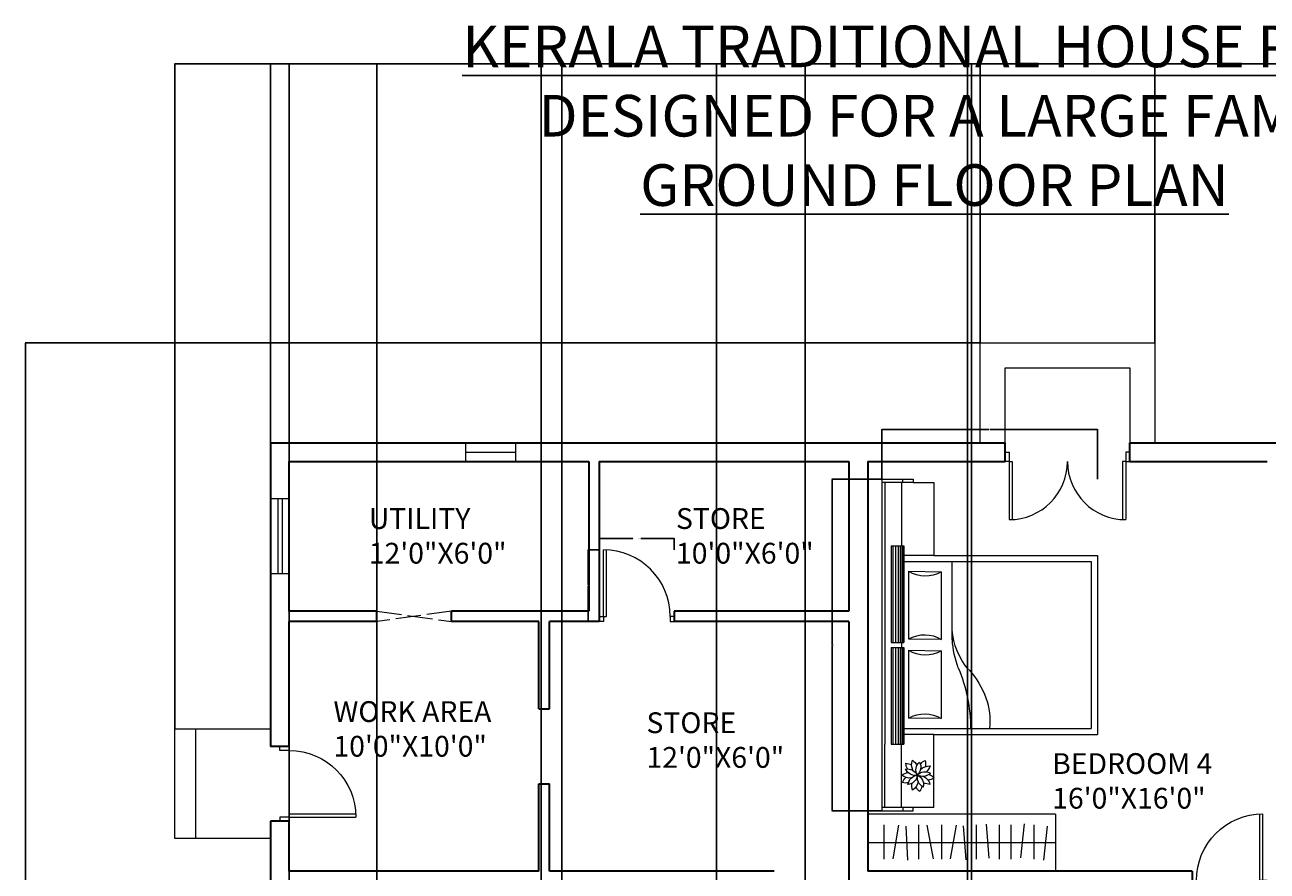
# Model space of a CAD drawing. Units: inches. Extents: x 4602 to 5612, y 5125 to 6591.
# Tile 5 of 6: x 4602 to 5199, y 6185 to 6591. Entities that reach past the tile are written whole.
import ezdxf

# ---------------------------------------------------------------- set-up
doc = ezdxf.new("R2010")
doc.units = ezdxf.units.IN
doc.linetypes.add('ACAD_ISO02W100', pattern=[15, 12, -3])
for name, color, linetype, lineweight in [('A-ANNO-DIMS', 2, 'Continuous', 18), ('A-ANNO-TEXT', 7, 'Continuous', 25), ('A-AREA-IDEN', 7, 'Continuous', 18), ('A-DOOR', 4, 'Continuous', 18), ('A-FLOR-CASE', 9, 'Continuous', 18), ('A-FLOR-STRS', 7, 'Continuous', 18), ('A-FURN', 8, 'Continuous', 13), ('A-GLAZ', 4, 'Continuous', 18), ('A-WALL', 7, 'Continuous', 35), ('A-WALL-OVHD', 8, 'ACAD_ISO02W100', 13)]:
    doc.layers.add(name, color=color, linetype=linetype, lineweight=lineweight)
doc.styles.get("Standard").update_dxf_attribs({"font": 'arial.ttf'})
doc.dimstyles.get("Standard").update_dxf_attribs({"dimtxt": 0.18, "dimasz": 0.18, "dimexe": 0.18, "dimexo": 0.0625, "dimgap": 0.09, "dimtad": 0, "dimtih": 1, "dimtoh": 1, "dimdec": 4, "dimzin": 0, "dimdsep": 46, "dimtxsty": 'Standard', "dimcen": 0.09, "dimadec": 0, "dimazin": 0, "dimtfac": 1, "dimtdec": 4, "dimtofl": 0, "dimtmove": 0, "dimatfit": 3, "dimfxl": 1, "dimtolj": 1, "dimtzin": 0, "dimarcsym": 0})

# ---------------------------------------------------------------- blocks, each defined once
blk = doc.blocks.new('A$C7BDD1693')
for p, q in [((0, 2.068), (0, 1.768)), ((0, 2.068), (1.615, 2.068)), ((0.03, 1.768), (0.03, 2.068)), ((0.03, 2.038), (0.64, 2.038)), ((0.64, 2.038), (1.565, 2.038)), ((1.565, 2.038), (1.615, 2.038)), ((1.615, 2.068), (2.54, 2.068)), ((1.615, 2.038), (2.54, 2.038)), ((2.54, 2.068), (3.18, 2.068)), ((3.15, 2.038), (2.54, 2.038)), ((3.15, 1.768), (3.15, 2.068)), ((3.18, 2.068), (3.18, 1.768)), ((0.64, 1.978), (1.565, 1.978)), ((0.64, 1.978), (0.64, 1.858)), ((0.64, 1.963), (1.565, 1.963)), ((0.64, 1.937), (1.565, 1.937)), ((0.64, 1.912), (1.565, 1.912)), ((1.565, 1.978), (1.565, 1.858)), ((1.615, 1.978), (1.615, 1.858)), ((1.615, 1.978), (2.54, 1.978)), ((1.615, 1.963), (2.54, 1.963)), ((1.615, 1.937), (2.54, 1.937)), ((1.615, 1.912), (2.54, 1.912)), ((2.54, 1.978), (2.54, 1.858)), ((0.03, 1.868), (0, 1.868)), ((0.03, 1.88), (0.64, 1.88)), ((0.64, 1.893), (1.565, 1.893)), ((0.64, 1.877), (1.565, 1.877)), ((0.64, 1.866), (1.565, 1.866)), ((0.64, 1.858), (1.565, 1.858)), ((0.73, 1.568), (0.73, 1.858)), ((0.79, 1.858), (0.79, 0.06)), ((1.533, 1.81), (0.883, 1.81)), ((0.883, 1.81), (0.887, 1.498)), ((1.537, 1.498), (1.533, 1.81)), ((1.565, 1.88), (1.615, 1.88)), ((1.615, 1.893), (2.54, 1.893)), ((1.615, 1.877), (2.54, 1.877)), ((1.615, 1.866), (2.54, 1.866)), ((1.615, 1.858), (2.54, 1.858)), ((2.291, 1.81), (1.641, 1.81)), ((1.641, 1.81), (1.646, 1.498)), ((2.296, 1.498), (2.291, 1.81)), ((2.39, 1.858), (2.39, 0.06)), ((2.45, 1.568), (2.45, 1.858)), ((3.15, 1.88), (2.54, 1.88)), ((3.15, 1.868), (3.18, 1.868)), ((0, 1.768), (0.03, 1.768)), ((0.03, 1.768), (0.03, 1.568)), ((0.03, 1.768), (0.03, 1.568)), ((3.15, 1.568), (3.15, 1.768)), ((3.18, 1.768), (3.15, 1.768)), ((0.03, 1.568), (0.73, 1.568)), ((0.73, 1.568), (0.73, 0)), ((3.15, 1.568), (2.45, 1.568)), ((2.45, 1.568), (2.45, 0)), ((0.887, 1.498), (1.537, 1.498)), ((1.646, 1.498), (2.296, 1.498)), ((1.54, 1.392), (0.79, 1.392)), ((1.848, 1.209), (0.79, 1.209)), ((0.73, 0), (2.45, 0)), ((0.79, 0.06), (2.39, 0.06))]:
    blk.add_line(p, q)
for centre, radius, start, end in [((0.626, 1.65), 0.303, 329.8722, 31.8713), ((1.794, 1.658), 0.303, 149.8722, 211.8713), ((1.384, 1.65), 0.303, 329.8722, 31.8713), ((2.553, 1.658), 0.303, 149.8722, 211.8713), ((2.879, 1.849), 0.155, 184.2105, 205.3514), ((2.726, 1.74), 0.0968, 57.5086, 91.2476), ((2.884, 1.823), 0.106, 170.7761, 244.5159), ((2.743, 1.749), 0.098, 347.0447, 68.2473), ((2.938, 1.802), 0.125, 143.1301, 173.4932), ((2.751, 1.802), 0.115, 351.1324, 40.6013), ((2.944, 1.713), 0.106, 98.7761, 172.5159), ((2.83, 1.825), 0.098, 275.0447, 356.2473), ((2.967, 1.726), 0.155, 112.2105, 133.3514), ((2.817, 1.838), 0.0968, 345.5086, 19.2476), ((2.74, 1.667), 0.115, 63.1324, 112.6013), ((2.798, 1.845), 0.125, 215.1301, 245.4931), ((2.791, 1.624), 0.0968, 129.5086, 163.2476), ((2.788, 1.643), 0.098, 59.0447, 140.2473), ((2.761, 1.8), 0.106, 242.7761, 316.5159), ((2.865, 1.615), 0.115, 135.1324, 184.6013), ((2.903, 1.653), 0.098, 131.0447, 212.2473), ((2.745, 1.676), 0.106, 314.7761, 28.5159), ((2.858, 1.622), 0.106, 26.7761, 100.5159), ((2.929, 1.765), 0.098, 203.0447, 284.2473), ((2.883, 1.833), 0.115, 279.1324, 328.6013), ((2.802, 1.607), 0.125, 359.1301, 29.4932), ((2.941, 1.655), 0.125, 71.1301, 101.4931), ((2.937, 1.782), 0.0968, 273.5086, 307.2476), ((2.877, 1.605), 0.155, 40.2105, 61.3514), ((2.735, 1.803), 0.155, 256.2105, 277.3514), ((2.713, 1.725), 0.125, 287.1301, 317.4932), ((2.921, 1.65), 0.0968, 201.5086, 235.2476), ((2.953, 1.718), 0.115, 207.1324, 256.6013), ((2.734, 1.652), 0.155, 328.2105, 349.3514)]:
    blk.add_arc(centre, radius, start, end)
for centre, major_axis, ratio, start_param, end_param in [((1.413, 0.552), (0, -0.842), 0.84, 2.512571, 3.097265), ((1.474, 0.023), (0, -1.371), 0.84, 2.845884, 3.083884), ((2.394, 3.329), (0, -2.112), 0.84, -0.336035, -0.002349), ((2.261, 1.856), (0.259, -0.793), 0.868451, -0.988378, -0.183496)]:
    blk.add_ellipse(centre, major_axis=major_axis, ratio=ratio, start_param=start_param, end_param=end_param)
blk = doc.blocks.new('DOOR-PAIR-60IN')
for p, q in [((2, 4.5), (2, 32.5)), ((3.5, 4.5), (3.5, 32.46)), ((56.5, 4.5), (56.5, 32.46)), ((58, 4.5), (58, 32.5)), ((2, 4.5), (0, 4.5)), ((2, 0), (2, 4.5)), ((2, 4.5), (3.5, 4.5)), ((58, 4.5), (56.5, 4.5)), ((58, 0), (58, 4.5)), ((58, 4.5), (60, 4.5)), ((0, 0), (2, 0)), ((60, 0), (58, 0))]:
    blk.add_line(p, q)
for centre, start, end in [((2, 4.5), 0, 90), ((58, 4.5), 90, 180)]:
    blk.add_arc(centre, 28, start, end)
blk = doc.blocks.new('DOOR-36IN-DEEP-JAMB')
for p, q in [((2, 4.5), (2, 36.5)), ((3.5, 4.5), (3.5, 36.46)), ((0, 4.5), (2, 4.5)), ((2, 4.5), (2, 0)), ((2, 4.5), (3.5, 4.5)), ((36, 4.5), (34, 4.5)), ((34, 4.5), (34, 0)), ((2, 0), (0, 0)), ((34, 0), (36, 0))]:
    blk.add_line(p, q)
blk.add_arc((2, 4.5), 32, 0, 90)
blk = doc.blocks.new('DOOR-36IN-SHALLOW-JAMB')
for p, q in [((2, 2.5), (2, 34.5)), ((3.5, 2.5), (3.5, 34.46)), ((0, 2.5), (2, 2.5)), ((2, 2.5), (2, 0)), ((2, 2.5), (3.5, 2.5)), ((36, 2.5), (34, 2.5)), ((34, 2.5), (34, 0)), ((2, 0), (0, 0)), ((34, 0), (36, 0))]:
    blk.add_line(p, q)
blk.add_arc((2, 2.5), 32, 0, 90)
blk = doc.blocks.new('WARDROBE-RAIL')
for p, q in [((90.22, 0), (90.22, 27.46)), ((3.99, 5.88), (5.71, 22.16)), ((10.39, 5.25), (10.39, 21.62)), ((15.01, 4.71), (16.73, 21)), ((21.48, 5.25), (21.48, 21.62)), ((27.02, 5.25), (27.02, 21.62)), ((33.26, 4.83), (31.94, 21.15)), ((38.1, 5.25), (38.1, 21.62)), ((44.31, 5.72), (42.98, 22.05)), ((47.72, 5.36), (50.53, 21.49)), ((54.72, 5.25), (54.72, 21.62)), ((61.87, 5.4), (58.77, 21.48)), ((65.8, 5.25), (65.8, 21.62)), ((70.89, 22.2), (71.76, 5.85)), ((75.49, 5.36), (78.19, 21.52)), ((82.43, 5.25), (82.43, 21.62)), ((90.22, 13.73), (0, 13.73)), ((0, 0), (90.22, 0))]:
    blk.add_line(p, q)
blk = doc.blocks.new('*D25')
at = {"layer": 'A-ANNO-DIMS', "color": 0, "lineweight": -2, "transparency": 16777216}
for p, q in [((4878.24, 6339.11), (4878.24, 6344.63)), ((4878.42, 6344.45), (4894.27, 6344.45)), ((4914.06, 6344.45), (4898.21, 6344.45)), ((4914.24, 6339.11), (4914.24, 6344.63))]:
    blk.add_line(p, q, dxfattribs=at)
at = {"layer": 'A-ANNO-DIMS', "color": 0, "transparency": 16777216}
for points in [[(4878.42, 6344.48), (4878.42, 6344.42), (4878.24, 6344.45)], [(4914.06, 6344.48), (4914.06, 6344.42), (4914.24, 6344.45)]]:
    blk.add_solid(points, dxfattribs=at)
at = {"layer": 'Defpoints', "color": 0, "transparency": 16777216}
for p in [(4914.24, 6344.45), (4878.24, 6339.05), (4914.24, 6339.05)]:
    blk.add_point(p, dxfattribs=at)
at = {"layer": 'A-ANNO-DIMS', "color": 0, "transparency": 16777216, "insert": (4896.24, 6344.45), "char_height": 0.18, "attachment_point": 5}
blk.add_mtext('\\A1;SHALLOW-JAMB DOOR 36 TYP.', dxfattribs=at)
blk = doc.blocks.new('*D26')
at = {"layer": 'A-ANNO-DIMS', "color": 0, "lineweight": -2, "transparency": 16777216}
for p, q in [((4878.18, 6339.05), (4872.66, 6339.05)), ((4872.84, 6338.87), (4872.84, 6321.98)), ((4872.84, 6304.73), (4872.84, 6321.62)), ((4878.18, 6304.55), (4872.66, 6304.55))]:
    blk.add_line(p, q, dxfattribs=at)
at = {"layer": 'A-ANNO-DIMS', "color": 0, "transparency": 16777216}
for points in [[(4872.81, 6338.87), (4872.87, 6338.87), (4872.84, 6339.05)], [(4872.81, 6304.73), (4872.87, 6304.73), (4872.84, 6304.55)]]:
    blk.add_solid(points, dxfattribs=at)
at = {"layer": 'Defpoints', "color": 0, "transparency": 16777216}
for p in [(4872.84, 6339.05), (4878.24, 6339.05), (4878.24, 6304.55)]:
    blk.add_point(p, dxfattribs=at)
at = {"layer": 'A-ANNO-DIMS', "color": 0, "transparency": 16777216, "insert": (4872.84, 6321.8), "char_height": 0.18, "attachment_point": 5}
blk.add_mtext('\\A1;35 TYP.', dxfattribs=at)
blk = doc.blocks.new('*D35')
at = {"layer": 'A-ANNO-DIMS', "color": 0, "lineweight": -2, "transparency": 16777216}
for p, q in [((5013.97, 6372.98), (4989.94, 6372.98)), ((4990.12, 6372.8), (4990.12, 6293.47)), ((4990.12, 6213.77), (4990.12, 6293.1)), ((5013.97, 6213.59), (4989.94, 6213.59))]:
    blk.add_line(p, q, dxfattribs=at)
at = {"layer": 'A-ANNO-DIMS', "color": 0, "transparency": 16777216}
for points in [[(4990.09, 6372.8), (4990.15, 6372.8), (4990.12, 6372.98)], [(4990.09, 6213.77), (4990.15, 6213.77), (4990.12, 6213.59)]]:
    blk.add_solid(points, dxfattribs=at)
at = {"layer": 'Defpoints', "color": 0, "transparency": 16777216}
for p in [(5014.03, 6372.98), (4990.12, 6213.59), (5014.03, 6213.59)]:
    blk.add_point(p, dxfattribs=at)
at = {"layer": 'A-ANNO-DIMS', "color": 0, "transparency": 16777216, "insert": (4990.12, 6293.29), "char_height": 0.18, "attachment_point": 5}
blk.add_mtext('\\A1;BED GROUP 159', dxfattribs=at)
blk = doc.blocks.new('*D36')
at = {"layer": 'A-ANNO-DIMS', "color": 0, "lineweight": -2, "transparency": 16777216}
for p, q in [((5014.03, 6373.04), (5014.03, 6397.07)), ((5014.21, 6396.89), (5065.58, 6396.89)), ((5117.5, 6396.89), (5066.14, 6396.89)), ((5117.68, 6373.04), (5117.68, 6397.07))]:
    blk.add_line(p, q, dxfattribs=at)
at = {"layer": 'A-ANNO-DIMS', "color": 0, "transparency": 16777216}
for points in [[(5014.21, 6396.92), (5014.21, 6396.86), (5014.03, 6396.89)], [(5117.5, 6396.92), (5117.5, 6396.86), (5117.68, 6396.89)]]:
    blk.add_solid(points, dxfattribs=at)
at = {"layer": 'Defpoints', "color": 0, "transparency": 16777216}
for p in [(5014.03, 6396.89), (5014.03, 6372.98), (5117.68, 6372.98)]:
    blk.add_point(p, dxfattribs=at)
at = {"layer": 'A-ANNO-DIMS', "color": 0, "transparency": 16777216, "insert": (5065.86, 6396.89), "char_height": 0.18, "attachment_point": 5}
blk.add_mtext('\\A1;104', dxfattribs=at)
blk = doc.blocks.new('*D55')
at = {"layer": 'A-ANNO-DIMS', "color": 0, "lineweight": -2, "transparency": 16777216}
for p, q in [((4674.24, 6252.95), (4674.24, 6572.85)), ((4674.42, 6572.67), (5106.95, 6572.67)), ((5540.06, 6572.67), (5107.53, 6572.67)), ((5540.24, 6127.61), (5540.24, 6572.85))]:
    blk.add_line(p, q, dxfattribs=at)
at = {"layer": 'A-ANNO-DIMS', "color": 0, "transparency": 16777216}
for points in [[(4674.42, 6572.7), (4674.42, 6572.64), (4674.24, 6572.67)], [(5540.06, 6572.7), (5540.06, 6572.64), (5540.24, 6572.67)]]:
    blk.add_solid(points, dxfattribs=at)
at = {"layer": 'Defpoints', "color": 0, "transparency": 16777216}
for p in [(5540.24, 6572.67), (4674.24, 6252.89), (5540.24, 6127.55)]:
    blk.add_point(p, dxfattribs=at)
at = {"layer": 'A-ANNO-DIMS', "color": 0, "transparency": 16777216, "insert": (5107.24, 6572.67), "char_height": 0.18, "attachment_point": 5}
blk.add_mtext('\\A1;866', dxfattribs=at)
blk = doc.blocks.new('*D56')
at = {"layer": 'A-ANNO-DIMS', "color": 0, "lineweight": -2, "transparency": 16777216}
for p, q in [((5061.18, 6438.55), (4602.21, 6438.55)), ((4602.39, 6438.37), (4602.39, 5817.73)), ((4602.39, 5196.73), (4602.39, 5817.37)), ((5055.18, 5196.55), (4602.21, 5196.55))]:
    blk.add_line(p, q, dxfattribs=at)
at = {"layer": 'A-ANNO-DIMS', "color": 0, "transparency": 16777216}
for points in [[(4602.36, 6438.37), (4602.42, 6438.37), (4602.39, 6438.55)], [(4602.36, 5196.73), (4602.42, 5196.73), (4602.39, 5196.55)]]:
    blk.add_solid(points, dxfattribs=at)
at = {"layer": 'Defpoints', "color": 0, "transparency": 16777216}
for p in [(4602.39, 6438.55), (5061.24, 6438.55), (5055.24, 5196.55)]:
    blk.add_point(p, dxfattribs=at)
at = {"layer": 'A-ANNO-DIMS', "color": 0, "transparency": 16777216, "insert": (4602.39, 5817.55), "char_height": 0.18, "attachment_point": 5}
blk.add_mtext('\\A1;1242', dxfattribs=at)
blk = doc.blocks.new('*D59')
at = {"layer": 'A-ANNO-DIMS', "color": 0, "lineweight": -2, "transparency": 16777216}
for p, q in [((4977.24, 5908.61), (4977.24, 6572.85)), ((4977.42, 6572.67), (5016.82, 6572.67)), ((5056.97, 6572.67), (5017.57, 6572.67)), ((5057.15, 5908.61), (5057.15, 6572.85))]:
    blk.add_line(p, q, dxfattribs=at)
at = {"layer": 'A-ANNO-DIMS', "color": 0, "transparency": 16777216}
for points in [[(4977.42, 6572.7), (4977.42, 6572.64), (4977.24, 6572.67)], [(5056.97, 6572.7), (5056.97, 6572.64), (5057.15, 6572.67)]]:
    blk.add_solid(points, dxfattribs=at)
at = {"layer": 'Defpoints', "color": 0, "transparency": 16777216}
for p in [(5057.15, 6572.67), (4977.24, 5908.55), (5057.15, 5908.55)]:
    blk.add_point(p, dxfattribs=at)
at = {"layer": 'A-ANNO-DIMS', "color": 0, "transparency": 16777216, "insert": (5017.19, 6572.67), "char_height": 0.18, "attachment_point": 5}
blk.add_mtext('\\A1;79.91', dxfattribs=at)
blk = doc.blocks.new('*D60')
at = {"layer": 'A-ANNO-DIMS', "color": 0, "lineweight": -2, "transparency": 16777216}
for p, q in [((4934.59, 5248.61), (4934.59, 6572.85)), ((4934.77, 6572.67), (4994.46, 6572.67)), ((5055.06, 6572.67), (4995.37, 6572.67)), ((5055.24, 5248.61), (5055.24, 6572.85))]:
    blk.add_line(p, q, dxfattribs=at)
at = {"layer": 'A-ANNO-DIMS', "color": 0, "transparency": 16777216}
for points in [[(4934.77, 6572.7), (4934.77, 6572.64), (4934.59, 6572.67)], [(5055.06, 6572.7), (5055.06, 6572.64), (5055.24, 6572.67)]]:
    blk.add_solid(points, dxfattribs=at)
at = {"layer": 'Defpoints', "color": 0, "transparency": 16777216}
for p in [(5055.24, 6572.67), (4934.59, 5248.55), (5055.24, 5248.55)]:
    blk.add_point(p, dxfattribs=at)
at = {"layer": 'A-ANNO-DIMS', "color": 0, "transparency": 16777216, "insert": (4994.91, 6572.67), "char_height": 0.18, "attachment_point": 5}
blk.add_mtext('\\A1;120.65', dxfattribs=at)
blk = doc.blocks.new('*D62')
at = {"layer": 'A-ANNO-DIMS', "color": 0, "lineweight": -2, "transparency": 16777216}
for p, q in [((4729.24, 5886.61), (4729.24, 6572.85)), ((4729.42, 6572.67), (4750.02, 6572.67)), ((4771.06, 6572.67), (4750.46, 6572.67)), ((4771.24, 5886.61), (4771.24, 6572.85))]:
    blk.add_line(p, q, dxfattribs=at)
at = {"layer": 'A-ANNO-DIMS', "color": 0, "transparency": 16777216}
for points in [[(4729.42, 6572.7), (4729.42, 6572.64), (4729.24, 6572.67)], [(4771.06, 6572.7), (4771.06, 6572.64), (4771.24, 6572.67)]]:
    blk.add_solid(points, dxfattribs=at)
at = {"layer": 'Defpoints', "color": 0, "transparency": 16777216}
for p in [(4771.24, 6572.67), (4729.24, 5886.55), (4771.24, 5886.55)]:
    blk.add_point(p, dxfattribs=at)
at = {"layer": 'A-ANNO-DIMS', "color": 0, "transparency": 16777216, "insert": (4750.24, 6572.67), "char_height": 0.18, "attachment_point": 5}
blk.add_mtext('\\A1;42', dxfattribs=at)
blk = doc.blocks.new('*D63')
at = {"layer": 'A-ANNO-DIMS', "color": 0, "lineweight": -2, "transparency": 16777216}
for p, q in [((4850.24, 5876.61), (4850.24, 6572.85)), ((4850.42, 6572.67), (4855.03, 6572.67)), ((4860.06, 6572.67), (4855.45, 6572.67)), ((4860.24, 5876.61), (4860.24, 6572.85))]:
    blk.add_line(p, q, dxfattribs=at)
at = {"layer": 'A-ANNO-DIMS', "color": 0, "transparency": 16777216}
for points in [[(4850.42, 6572.7), (4850.42, 6572.64), (4850.24, 6572.67)], [(4860.06, 6572.7), (4860.06, 6572.64), (4860.24, 6572.67)]]:
    blk.add_solid(points, dxfattribs=at)
at = {"layer": 'Defpoints', "color": 0, "transparency": 16777216}
for p in [(4860.24, 6572.67), (4850.24, 5876.55), (4860.24, 5876.55)]:
    blk.add_point(p, dxfattribs=at)
at = {"layer": 'A-ANNO-DIMS', "color": 0, "transparency": 16777216, "insert": (4855.24, 6572.67), "char_height": 0.18, "attachment_point": 5}
blk.add_mtext('\\A1;10', dxfattribs=at)
blk = doc.blocks.new('*D67')
at = {"layer": 'A-ANNO-DIMS', "color": 0, "lineweight": -2, "transparency": 16777216}
for p, q in [((5061.24, 6438.61), (5061.24, 6572.85)), ((5061.42, 6572.67), (5103.02, 6572.67)), ((5145.06, 6572.67), (5103.46, 6572.67)), ((5145.24, 6438.61), (5145.24, 6572.85))]:
    blk.add_line(p, q, dxfattribs=at)
at = {"layer": 'A-ANNO-DIMS', "color": 0, "transparency": 16777216}
for points in [[(5061.42, 6572.7), (5061.42, 6572.64), (5061.24, 6572.67)], [(5145.06, 6572.7), (5145.06, 6572.64), (5145.24, 6572.67)]]:
    blk.add_solid(points, dxfattribs=at)
at = {"layer": 'Defpoints', "color": 0, "transparency": 16777216}
for p in [(5145.24, 6572.67), (5061.24, 6438.55), (5145.24, 6438.55)]:
    blk.add_point(p, dxfattribs=at)
at = {"layer": 'A-ANNO-DIMS', "color": 0, "transparency": 16777216, "insert": (5103.24, 6572.67), "char_height": 0.18, "attachment_point": 5}
blk.add_mtext('\\A1;84', dxfattribs=at)
blk = doc.blocks.new('*D69')
at = {"layer": 'A-ANNO-DIMS', "color": 0, "lineweight": -2, "transparency": 16777216}
for p, q in [((4674.24, 6252.95), (4674.24, 6572.85)), ((4674.42, 6572.67), (4697.02, 6572.67)), ((4720.06, 6572.67), (4697.46, 6572.67)), ((4720.24, 6252.95), (4720.24, 6572.85))]:
    blk.add_line(p, q, dxfattribs=at)
at = {"layer": 'A-ANNO-DIMS', "color": 0, "transparency": 16777216}
for points in [[(4674.42, 6572.7), (4674.42, 6572.64), (4674.24, 6572.67)], [(4720.06, 6572.7), (4720.06, 6572.64), (4720.24, 6572.67)]]:
    blk.add_solid(points, dxfattribs=at)
at = {"layer": 'Defpoints', "color": 0, "transparency": 16777216}
for p in [(4720.24, 6572.67), (4674.24, 6252.89), (4720.24, 6252.89)]:
    blk.add_point(p, dxfattribs=at)
at = {"layer": 'A-ANNO-DIMS', "color": 0, "transparency": 16777216, "insert": (4697.24, 6572.67), "char_height": 0.18, "attachment_point": 5}
blk.add_mtext('\\A1;46', dxfattribs=at)
blk = doc.blocks.new('*D71')
at = {"layer": 'A-ANNO-DIMS', "color": 0, "lineweight": -2, "transparency": 16777216}
for p, q in [((4720.24, 6390.61), (4720.24, 6572.85)), ((4720.42, 6572.67), (4724.59, 6572.67)), ((4729.06, 6572.67), (4724.89, 6572.67)), ((4729.24, 6381.61), (4729.24, 6572.85))]:
    blk.add_line(p, q, dxfattribs=at)
at = {"layer": 'A-ANNO-DIMS', "color": 0, "transparency": 16777216}
for points in [[(4720.42, 6572.7), (4720.42, 6572.64), (4720.24, 6572.67)], [(4729.06, 6572.7), (4729.06, 6572.64), (4729.24, 6572.67)]]:
    blk.add_solid(points, dxfattribs=at)
at = {"layer": 'Defpoints', "color": 0, "transparency": 16777216}
for p in [(4729.24, 6572.67), (4720.24, 6390.55), (4729.24, 6381.55)]:
    blk.add_point(p, dxfattribs=at)
at = {"layer": 'A-ANNO-DIMS', "color": 0, "transparency": 16777216, "insert": (4724.74, 6572.67), "char_height": 0.18, "attachment_point": 5}
blk.add_mtext('\\A1;9', dxfattribs=at)

msp = doc.modelspace()

# ---------------------------------------------------------------- linework, layer by layer
at = {"layer": 'A-FLOR-CASE'}
msp.add_line((5097.4613, 6212.0089), (5097.4613, 6184.5515), dxfattribs=at)
at = {"layer": 'A-FLOR-STRS'}
for p, q in [((5061.239, 6390.5515), (5061.239, 6438.5515)), ((5061.239, 6438.5515), (5145.239, 6438.5515)), ((5145.239, 6438.5515), (5145.239, 6390.5515)), ((5073.239, 6390.5515), (5073.239, 6426.5515)), ((5073.239, 6426.5515), (5133.239, 6426.5515)), ((5133.239, 6426.5515), (5133.239, 6390.5515)), ((4720.239, 6252.8852), (4674.239, 6252.8852)), ((4674.239, 6200.2515), (4674.239, 6252.8852)), ((4684.239, 6200.2515), (4684.239, 6252.8852)), ((4720.239, 6200.2515), (4674.239, 6200.2515))]:
    msp.add_line(p, q, dxfattribs=at)
at = {"layer": 'A-GLAZ'}
for p, q in [((4814.0792, 6381.5515), (4814.0792, 6390.5515)), ((4838.0792, 6381.5515), (4838.0792, 6390.5515)), ((4814.0792, 6386.0515), (4838.0792, 6386.0515)), ((4729.239, 6363.5515), (4720.239, 6363.5515)), ((4723.739, 6363.5515), (4723.739, 6327.5515)), ((4725.739, 6363.5515), (4725.739, 6327.5515)), ((4729.239, 6327.5515), (4720.239, 6327.5515))]:
    msp.add_line(p, q, dxfattribs=at)
at = {"layer": 'A-WALL'}
for p, q in [((4720.239, 6390.5515), (5073.239, 6390.5515)), ((4720.239, 6390.5515), (4720.239, 6244.5515)), ((5073.239, 6381.5515), (5073.239, 6390.5515)), ((5133.239, 6381.5515), (5133.239, 6390.5515)), ((5133.239, 6390.5515), (5486.239, 6390.5515)), ((4729.239, 6381.5515), (4873.239, 6381.5515)), ((4729.239, 6309.5515), (4729.239, 6381.5515)), ((4873.239, 6381.5515), (4873.239, 6309.5515)), ((4878.239, 6381.5515), (4878.239, 6304.5515)), ((4878.239, 6381.5515), (4998.239, 6381.5515)), ((4998.239, 6381.5515), (4998.239, 6309.5515)), ((5007.239, 6381.5515), (5007.239, 6184.5515)), ((5007.239, 6381.5515), (5073.239, 6381.5515)), ((5133.239, 6381.5515), (5199.239, 6381.5515)), ((4771.239, 6309.5515), (4729.239, 6309.5515)), ((4771.239, 6304.5515), (4771.239, 6309.5515)), ((4873.239, 6309.5515), (4807.239, 6309.5515)), ((4807.239, 6304.5515), (4807.239, 6309.5515)), ((4998.239, 6309.5515), (4914.239, 6309.5515)), ((4914.239, 6309.5515), (4914.239, 6304.5515)), ((4771.239, 6304.5515), (4729.239, 6304.5515)), ((4729.239, 6244.5515), (4729.239, 6304.5515)), ((4849.239, 6304.5515), (4807.239, 6304.5515)), ((4849.239, 6262.5515), (4849.239, 6304.5515)), ((4878.239, 6304.5515), (4854.239, 6304.5515)), ((4854.239, 6262.5515), (4854.239, 6304.5515)), ((4998.239, 6304.5515), (4914.239, 6304.5515)), ((4998.239, 6304.5515), (4998.239, 6175.5515)), ((4849.239, 6262.5515), (4854.239, 6262.5515)), ((4729.239, 6244.5515), (4720.239, 6244.5515)), ((4849.239, 6184.5515), (4849.239, 6226.5515)), ((4849.239, 6226.5515), (4854.239, 6226.5515)), ((4854.239, 6184.5515), (4854.239, 6226.5515)), ((4729.239, 6208.5515), (4720.239, 6208.5515)), ((4720.239, 6208.5515), (4720.239, 5380.5515)), ((4729.239, 6184.5515), (4729.239, 6208.5515)), ((4849.239, 6184.5515), (4729.239, 6184.5515)), ((4962.239, 6184.5515), (4854.239, 6184.5515)), ((5163.239, 6184.5515), (5007.239, 6184.5515)), ((5163.239, 6184.5515), (5163.239, 6175.5515))]:
    msp.add_line(p, q, dxfattribs=at)
at = {"layer": 'A-WALL-OVHD'}
for p, q in [((4807.239, 6309.5515), (4771.239, 6304.5515)), ((4771.239, 6309.5515), (4807.239, 6304.5515))]:
    msp.add_line(p, q, dxfattribs=at)

# ---------------------------------------------------------------- block references
at = {"layer": 'A-DOOR', "rotation": 180}
msp.add_blockref('DOOR-PAIR-60IN', (5133.2391, 6386.051), dxfattribs=at)
at = {"layer": 'A-DOOR'}
msp.add_blockref('DOOR-36IN-SHALLOW-JAMB', (4878.239, 6304.552), dxfattribs=at)
at = {"layer": 'A-DOOR', "extrusion": (0, 0, -1), "zscale": -1, "rotation": 89.99999999999781}
msp.add_blockref('DOOR-36IN-DEEP-JAMB', (-4724.7395, 6208.5515), dxfattribs=at)
at = {"layer": 'A-DOOR', "extrusion": (0, 0, -1), "zscale": -1}
msp.add_blockref('DOOR-36IN-DEEP-JAMB', (-5199.2391, 6175.552), dxfattribs=at)
at = {"layer": 'A-FLOR-CASE', "rotation": 180}
msp.add_blockref('WARDROBE-RAIL', (5097.4614, 6212.009), dxfattribs=at)
at = {"layer": 'A-FURN', "xscale": -50.12329360170435, "yscale": 50.12329360170435, "zscale": 50.12329360170435, "rotation": 90}
msp.add_blockref('A$C7BDD1693', (5117.6811, 6372.9816), dxfattribs=at)

# ---------------------------------------------------------------- texts
at = {"layer": 'A-ANNO-TEXT', "insert": (4812.35, 6591.1079), "char_height": 20, "attachment_point": 1}
msp.add_mtext_dynamic_manual_height_columns('{\\LKERALA TRADITIONAL HOUSE PLAN 2000 SQFT \\P}      DESIGNED FOR A LARGE FAMILY\\P              {\\LGROUND FLOOR PLAN}', width=869.722344, gutter_width=12.5, heights=[0], dxfattribs=at)
at = {"layer": 'A-AREA-IDEN', "char_height": 10, "attachment_point": 1}
for s, width, insert in [('UTILITY \\P12\'0"X6\'0"', 54.473105, (4767.4437, 6359.0908)), ('STORE\\P10\'0"X6\'0"', 54.473105, (4915.088, 6359.0908)), ('WORK AREA\\P10\'0"X10\'0"', 140.595401, (4750.4354, 6266.2782)), ('STORE\\P12\'0"X6\'0"', 54.473105, (4900.8979, 6260.9081)), ('BEDROOM 4\\P16\'0"X16\'0"', 88.287986, (5095.9036, 6241.2801))]:
    msp.add_mtext_dynamic_manual_height_columns(s, width=width, gutter_width=12.5, heights=[0], dxfattribs=dict(at, insert=insert))

# ---------------------------------------------------------------- dimensions: what is measured, and where the dimension line sits
at = {"layer": 'A-ANNO-DIMS'}
for base, p1, p2, override, picture, middle in [((5540.239, 6572.6716), (4674.239, 6252.8852), (5540.239, 6127.5515), {"dimdec": 0, "dimlfac": 1, "dimrnd": 0, "dimzin": 0, "dimdsep": 46, "dimlunit": 2}, '*D55', (5107.239, 6572.6716)), ((4720.239, 6572.6716), (4674.239, 6252.8852), (4720.239, 6252.8852), {"dimdec": 0, "dimlfac": 1, "dimrnd": 0, "dimzin": 0, "dimdsep": 46, "dimlunit": 2}, '*D69', (4697.239, 6572.6716)), ((4729.239, 6572.6716), (4720.239, 6390.5515), (4729.239, 6381.5515), {"dimdec": 0, "dimlfac": 1, "dimrnd": 0, "dimzin": 0, "dimdsep": 46, "dimlunit": 2}, '*D71', (4724.739, 6572.6716)), ((4771.239, 6572.6716), (4729.239, 5886.5515), (4771.239, 5886.5515), {"dimdec": 0, "dimlfac": 1, "dimrnd": 0, "dimzin": 0, "dimdsep": 46, "dimlunit": 2}, '*D62', (4750.239, 6572.6716)), ((4860.239, 6572.6716), (4850.239, 5876.5515), (4860.239, 5876.5515), {"dimdec": 0, "dimlfac": 1, "dimrnd": 0, "dimzin": 0, "dimdsep": 46, "dimlunit": 2}, '*D63', (4855.239, 6572.6716)), ((5055.239, 6572.6716), (4934.5878, 5248.5515), (5055.239, 5248.5515), {"dimdec": 2, "dimlfac": 1, "dimrnd": 0, "dimzin": 0, "dimdsep": 46, "dimlunit": 2}, '*D60', (4994.9134, 6572.6716)), ((5057.1497, 6572.6716), (4977.239, 5908.5515), (5057.1497, 5908.5515), {"dimdec": 2, "dimlfac": 1, "dimrnd": 0, "dimzin": 0, "dimdsep": 46, "dimlunit": 2}, '*D59', (5017.1944, 6572.6716)), ((5145.239, 6572.6716), (5061.239, 6438.5515), (5145.239, 6438.5515), {"dimdec": 0, "dimlfac": 1, "dimrnd": 0, "dimzin": 0, "dimdsep": 46, "dimlunit": 2}, '*D67', (5103.239, 6572.6716))]:
    dim = msp.add_linear_dim(base=base, p1=p1, p2=p2, dimstyle='Standard', override=override, dxfattribs=at)
    dim.commit()
    dim.dimension.update_dxf_attribs({"geometry": picture, "text_midpoint": middle})
for base, p1, p2, angle, picture, middle in [((4602.389, 6438.5515), (5055.239, 5196.5515), (5061.239, 6438.5515), 90, '*D56', (4602.389, 5817.5515)), ((5014.0319, 6396.8904), (5117.6811, 6372.9816), (5014.0319, 6372.9816), 180, '*D36', (5065.8565, 6396.8904))]:
    dim = msp.add_linear_dim(base=base, p1=p1, p2=p2, angle=angle, dimstyle='Standard', override={"dimdec": 0, "dimlfac": 1, "dimrnd": 0, "dimzin": 0, "dimdsep": 46, "dimlunit": 2}, dxfattribs=at)
    dim.commit()
    dim.dimension.update_dxf_attribs({"geometry": picture, "text_midpoint": middle})
for base, p1, p2, angle, text, picture, middle in [((4990.1231, 6213.5896), (5014.0319, 6372.9816), (5014.0319, 6213.5896), 270, 'BED GROUP <>', '*D35', (4990.1231, 6293.2856)), ((4872.8390416823, 6339.0515203146), (4878.2390416823, 6304.5515203146), (4878.2390416823, 6339.0515203146), 90, '<> TYP.', '*D26', (4872.8390416823, 6321.8015203146))]:
    dim = msp.add_linear_dim(base=base, p1=p1, p2=p2, angle=angle, text=text, dimstyle='Standard', override={"dimdec": 0, "dimlfac": 1, "dimrnd": 0, "dimzin": 0, "dimdsep": 46, "dimlunit": 2}, dxfattribs=at)
    dim.commit()
    dim.dimension.update_dxf_attribs({"geometry": picture, "text_midpoint": middle})
dim = msp.add_linear_dim(base=(4914.239, 6344.4515), p1=(4878.239, 6339.0515), p2=(4914.239, 6339.0515), text='SHALLOW-JAMB DOOR <> TYP.', dimstyle='Standard', override={"dimdec": 0, "dimlfac": 1, "dimrnd": 0, "dimzin": 0, "dimdsep": 46, "dimlunit": 2}, dxfattribs=at)
dim.commit()
dim.dimension.update_dxf_attribs({"geometry": '*D25', "text_midpoint": (4896.239, 6344.4515)})

doc.saveas('drawing.dxf')
